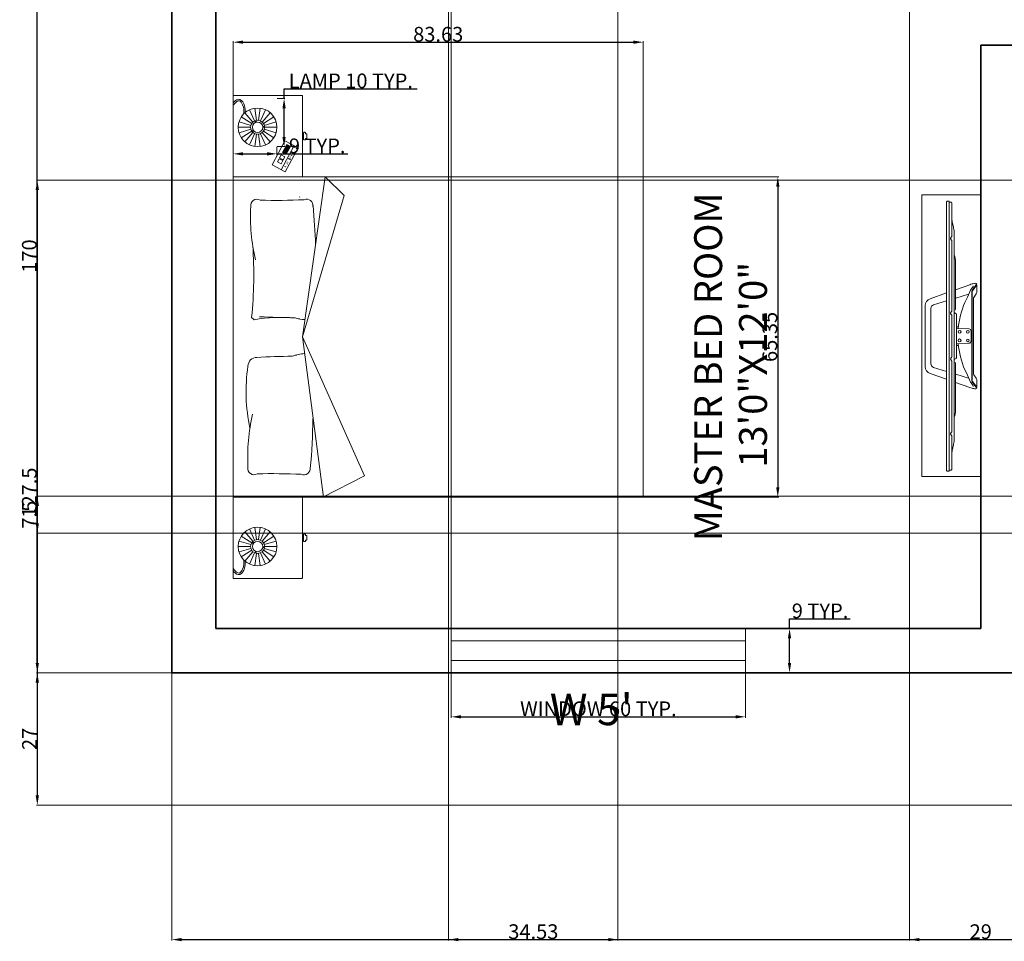
# Model space of a CAD drawing. Units: feet. Extents: x -297 to 770, y -228 to 625.
# Tile 1 of 14: x 351 to 552, y -228 to -40. Entities that reach past the tile are written whole.
import ezdxf

# ---------------------------------------------------------------- set-up
doc = ezdxf.new("R2010")
doc.units = ezdxf.units.FT
doc.header["$MEASUREMENT"] = 0
for name, color, linetype, lineweight in [('A-ANNO-DIMS', 2, 'Continuous', 18), ('A-ANNO-TEXT', 7, 'Continuous', 18), ('A-AREA-IDEN', 7, 'Continuous', 25), ('A-EQPM', 8, 'Continuous', 13), ('A-FURN', 8, 'Continuous', 18), ('A-WALL', 7, 'Continuous', 35), ('windows', 30, 'Continuous', 18)]:
    doc.layers.add(name, color=color, linetype=linetype, lineweight=lineweight)
doc.styles.add('Annotative', font='arial.ttf')
doc.styles.get("Standard").update_dxf_attribs({"font": 'arial.ttf'})
doc.dimstyles.get("Standard").update_dxf_attribs({"dimtxt": 3, "dimasz": 2, "dimexe": 0.18, "dimexo": 0.0625, "dimgap": 0.09, "dimtad": 1, "dimtoh": 1, "dimdec": 1, "dimzin": 0, "dimdsep": 46, "dimlunit": 3, "dimtxsty": 'Standard', "dimcen": 0, "dimclre": 256, "dimadec": 0, "dimazin": 0, "dimtfac": 1, "dimtdec": 1, "dimtofl": 0, "dimtmove": 0, "dimatfit": 3, "dimfxl": 1, "dimtolj": 1, "dimtzin": 0, "dimlwe": -1, "dimarcsym": 0})

# ---------------------------------------------------------------- blocks, each defined once
blk = doc.blocks.new('WIN-5FT')
for p, q in [((60, 6.5), (0, 6.5)), ((60, 2.5), (0, 2.5))]:
    blk.add_line(p, q)
blk.add_lwpolyline([(60, 0), (60, 9), (0, 9), (0, 0)], close=True)
blk = doc.blocks.new('LAMP-BEDSIDE')
for p, q in [((1.64, 6.07), (3.76, 4.71)), ((2.38, 6.92), (4.02, 5.02)), ((3.32, 7.53), (4.37, 5.24)), ((4.4, 7.84), (4.76, 5.35)), ((5.52, 7.84), (5.16, 5.35)), ((6.6, 7.53), (5.55, 5.24)), ((7.54, 6.92), (5.89, 5.02)), ((8.27, 6.07), (6.16, 4.71)), ((1.18, 5.05), (3.59, 4.34)), ((4.52, 4.9), (4.45, 5.28)), ((4.73, 4.97), (4.58, 5.32)), ((6, 4.13), (6.37, 4.13)), ((6.33, 4.34), (8.74, 5.05)), ((1.02, 3.94), (3.53, 3.94)), ((1.02, 3.94), (3.53, 3.94)), ((1.18, 2.83), (3.59, 3.54)), ((3.76, 3.17), (1.64, 1.81)), ((4.02, 2.86), (2.38, 0.96)), ((4.37, 2.64), (3.32, 0.36)), ((4.06, 3.38), (3.84, 3.06)), ((4.29, 3.12), (3.96, 2.92)), ((4.76, 2.53), (4.4, 0.04)), ((5.16, 2.53), (5.52, 0.04)), ((5.55, 2.64), (6.6, 0.36)), ((5.89, 2.86), (7.54, 0.96)), ((6.02, 3.89), (6.39, 3.98)), ((6.16, 3.17), (8.27, 1.81)), ((6.33, 3.54), (8.74, 2.83)), ((6.39, 3.94), (8.9, 3.94)), ((6.39, 3.94), (8.9, 3.94))]:
    blk.add_line(p, q)
for radius in [3.94, 1.43, 1.06]:
    blk.add_circle((4.96, 3.94), radius)
for points, knots in [([(2.46, 6.99), (2.46, 7.42), (2.45, 7.88), (2.14, 8.85), (1.91, 9.46), (0.86, 9.79), (0.47, 9.43), (0.1, 9.02), (0.05, 8.96), (0, 8.91)], [0.0077183, 0.0077183, 0.0077183, 0.0077183, 0.0428867, 0.0428867, 0.0785443, 0.0785443, 0.1084778, 0.1084778, 0.1132873, 0.1132873, 0.1132873, 0.1132873]), ([(2.16, 6.71), (2.17, 7.31), (2.19, 8.25), (1.15, 9.83), (0.43, 8.96), (0, 8.44)], [0, 0, 0, 0, 1.847824, 2.900884, 4.449581, 4.449581, 4.449581, 4.449581])]:
    blk.add_open_spline(points, degree=3, knots=knots)
blk = doc.blocks.new('*D19')
at = {"layer": 'A-ANNO-DIMS', "transparency": 16777216}
for p, q in [((439.16, -173.1), (439.16, -182.22)), ((499.16, -173.1), (499.16, -182.22))]:
    blk.add_line(p, q, dxfattribs=at)
at = {"layer": 'A-ANNO-DIMS', "color": 0, "lineweight": -2, "transparency": 16777216}
blk.add_line((441.16, -182.04), (497.16, -182.04), dxfattribs=at)
at = {"layer": 'A-ANNO-DIMS', "color": 0, "transparency": 16777216}
for points in [[(441.16, -181.7), (441.16, -182.37), (439.16, -182.04)], [(497.16, -181.7), (497.16, -182.37), (499.16, -182.04)]]:
    blk.add_solid(points, dxfattribs=at)
at = {"layer": 'Defpoints', "color": 0, "transparency": 16777216}
for p in [(439.16, -173.04), (499.16, -173.04), (499.16, -182.04)]:
    blk.add_point(p, dxfattribs=at)
at = {"layer": 'A-ANNO-DIMS', "color": 0, "transparency": 16777216, "insert": (469.16, -180.4), "char_height": 3, "attachment_point": 5}
blk.add_mtext('\\A1;WINDOW 60 TYP.', dxfattribs=at)
blk = doc.blocks.new('*D20')
at = {"layer": 'A-ANNO-DIMS', "color": 0, "lineweight": -2, "transparency": 16777216}
for p, q in [((508.16, -164.04), (508.16, -162.04)), ((508.16, -162.04), (520.52, -162.04)), ((508.16, -171.04), (508.16, -166.04))]:
    blk.add_line(p, q, dxfattribs=at)
at = {"layer": 'A-ANNO-DIMS', "transparency": 16777216}
for p, q in [((499.22, -164.04), (508.34, -164.04)), ((499.22, -173.04), (508.34, -173.04))]:
    blk.add_line(p, q, dxfattribs=at)
at = {"layer": 'A-ANNO-DIMS', "color": 0, "transparency": 16777216}
for points in [[(507.82, -166.04), (508.49, -166.04), (508.16, -164.04)], [(507.82, -171.04), (508.49, -171.04), (508.16, -173.04)]]:
    blk.add_solid(points, dxfattribs=at)
at = {"layer": 'Defpoints', "color": 0, "transparency": 16777216}
for p in [(499.16, -164.04), (508.16, -164.04), (499.16, -173.04)]:
    blk.add_point(p, dxfattribs=at)
at = {"layer": 'A-ANNO-DIMS', "color": 0, "transparency": 16777216, "insert": (514.38, -160.42), "char_height": 3, "attachment_point": 5}
blk.add_mtext('\\A1;9 TYP.', dxfattribs=at)
blk = doc.blocks.new('*D25')
at = {"layer": 'A-ANNO-DIMS', "color": 0, "lineweight": -2, "transparency": 16777216}
for p, q in [((405.05, -55.92), (405.05, -53.92)), ((405.05, -53.92), (432.18, -53.92)), ((405.05, -63.72), (405.05, -57.92))]:
    blk.add_line(p, q, dxfattribs=at)
at = {"layer": 'A-ANNO-DIMS', "transparency": 16777216}
for p, q in [((403.64, -55.92), (405.23, -55.92)), ((403.64, -65.72), (405.23, -65.72))]:
    blk.add_line(p, q, dxfattribs=at)
at = {"layer": 'A-ANNO-DIMS', "color": 0, "transparency": 16777216}
for points in [[(404.71, -57.92), (405.38, -57.92), (405.05, -55.92)], [(404.71, -63.72), (405.38, -63.72), (405.05, -65.72)]]:
    blk.add_solid(points, dxfattribs=at)
at = {"layer": 'Defpoints', "color": 0, "transparency": 16777216}
for p in [(403.58, -55.92), (405.05, -55.92), (403.58, -65.72)]:
    blk.add_point(p, dxfattribs=at)
at = {"layer": 'A-ANNO-DIMS', "color": 0, "transparency": 16777216, "insert": (418.66, -52.3), "char_height": 3, "attachment_point": 5}
blk.add_mtext('\\A1;LAMP 10 TYP.', dxfattribs=at)
blk = doc.blocks.new('*D26')
at = {"layer": 'A-ANNO-DIMS', "transparency": 16777216}
for p, q in [((394.68, -65.78), (394.68, -67.37)), ((403.58, -65.78), (403.58, -67.37))]:
    blk.add_line(p, q, dxfattribs=at)
at = {"layer": 'A-ANNO-DIMS', "color": 0, "lineweight": -2, "transparency": 16777216}
for p, q in [((396.68, -67.19), (401.58, -67.19)), ((403.58, -67.19), (418.03, -67.19))]:
    blk.add_line(p, q, dxfattribs=at)
at = {"layer": 'A-ANNO-DIMS', "color": 0, "transparency": 16777216}
for points in [[(396.68, -66.85), (396.68, -67.52), (394.68, -67.19)], [(401.58, -66.85), (401.58, -67.52), (403.58, -67.19)]]:
    blk.add_solid(points, dxfattribs=at)
at = {"layer": 'Defpoints', "color": 0, "transparency": 16777216}
for p in [(394.68, -65.72), (403.58, -65.72), (403.58, -67.19)]:
    blk.add_point(p, dxfattribs=at)
at = {"layer": 'A-ANNO-DIMS', "color": 0, "transparency": 16777216, "insert": (411.8, -65.56), "char_height": 3, "attachment_point": 5}
blk.add_mtext('\\A1;9 TYP.', dxfattribs=at)
blk = doc.blocks.new('*D43')
at = {"layer": 'A-ANNO-DIMS', "transparency": 16777216}
for p, q in [((382.16, -173.1), (382.16, -227.67)), ((742.16, -200.1), (742.16, -227.67))]:
    blk.add_line(p, q, dxfattribs=at)
at = {"layer": 'A-ANNO-DIMS', "color": 0, "lineweight": -2, "transparency": 16777216}
blk.add_line((384.16, -227.49), (740.16, -227.49), dxfattribs=at)
at = {"layer": 'A-ANNO-DIMS', "color": 0, "transparency": 16777216}
for points in [[(384.16, -227.15), (384.16, -227.82), (382.16, -227.49)], [(740.16, -227.15), (740.16, -227.82), (742.16, -227.49)]]:
    blk.add_solid(points, dxfattribs=at)
at = {"layer": 'Defpoints', "color": 0, "transparency": 16777216}
for p in [(382.16, -173.04), (742.16, -200.04), (742.16, -227.49)]:
    blk.add_point(p, dxfattribs=at)
at = {"layer": 'A-ANNO-DIMS', "color": 0, "transparency": 16777216, "insert": (562.16, -225.86), "char_height": 3, "attachment_point": 5}
blk.add_mtext('\\A1;360', dxfattribs=at)
blk = doc.blocks.new('*D45')
at = {"layer": 'A-ANNO-DIMS', "transparency": 16777216}
for p, q in [((382.09, -173.04), (354.53, -173.04)), ((556.09, -200.04), (354.53, -200.04))]:
    blk.add_line(p, q, dxfattribs=at)
at = {"layer": 'A-ANNO-DIMS', "color": 0, "lineweight": -2, "transparency": 16777216}
blk.add_line((354.71, -175.04), (354.71, -198.04), dxfattribs=at)
at = {"layer": 'A-ANNO-DIMS', "color": 0, "transparency": 16777216}
for points in [[(354.37, -175.04), (355.04, -175.04), (354.71, -173.04)], [(354.37, -198.04), (355.04, -198.04), (354.71, -200.04)]]:
    blk.add_solid(points, dxfattribs=at)
at = {"layer": 'Defpoints', "color": 0, "transparency": 16777216}
for p in [(382.16, -173.04), (354.71, -200.04), (556.16, -200.04)]:
    blk.add_point(p, dxfattribs=at)
at = {"layer": 'A-ANNO-DIMS', "color": 0, "transparency": 16777216, "insert": (353.11, -186.54), "char_height": 3, "attachment_point": 5, "rotation": 90}
blk.add_mtext('\\A1;27', dxfattribs=at)
blk = doc.blocks.new('*D53')
at = {"layer": 'A-ANNO-DIMS', "transparency": 16777216}
for p, q in [((382.09, -3.04), (354.53, -3.04)), ((382.09, -173.04), (354.53, -173.04))]:
    blk.add_line(p, q, dxfattribs=at)
at = {"layer": 'A-ANNO-DIMS', "color": 0, "lineweight": -2, "transparency": 16777216}
blk.add_line((354.71, -171.04), (354.71, -5.04), dxfattribs=at)
at = {"layer": 'A-ANNO-DIMS', "color": 0, "transparency": 16777216}
for points in [[(354.37, -5.04), (355.04, -5.04), (354.71, -3.04)], [(354.37, -171.04), (355.04, -171.04), (354.71, -173.04)]]:
    blk.add_solid(points, dxfattribs=at)
at = {"layer": 'Defpoints', "color": 0, "transparency": 16777216}
for p in [(354.71, -3.04), (382.16, -3.04), (382.16, -173.04)]:
    blk.add_point(p, dxfattribs=at)
at = {"layer": 'A-ANNO-DIMS', "color": 0, "transparency": 16777216, "insert": (353.08, -88.04), "char_height": 3, "attachment_point": 5, "rotation": 90}
blk.add_mtext('\\A1;170', dxfattribs=at)
blk = doc.blocks.new('*D56')
at = {"layer": 'A-ANNO-DIMS', "transparency": 16777216}
for p, q in [((742.09, -72.54), (354.53, -72.54)), ((742.09, -200.04), (354.53, -200.04))]:
    blk.add_line(p, q, dxfattribs=at)
at = {"layer": 'A-ANNO-DIMS', "color": 0, "lineweight": -2, "transparency": 16777216}
blk.add_line((354.71, -74.54), (354.71, -198.04), dxfattribs=at)
at = {"layer": 'A-ANNO-DIMS', "color": 0, "transparency": 16777216}
for points in [[(354.37, -74.54), (355.04, -74.54), (354.71, -72.54)], [(354.37, -198.04), (355.04, -198.04), (354.71, -200.04)]]:
    blk.add_solid(points, dxfattribs=at)
at = {"layer": 'Defpoints', "color": 0, "transparency": 16777216}
for p in [(742.16, -72.54), (354.71, -200.04), (742.16, -200.04)]:
    blk.add_point(p, dxfattribs=at)
at = {"layer": 'A-ANNO-DIMS', "color": 0, "transparency": 16777216, "insert": (353.08, -136.29), "char_height": 3, "attachment_point": 5, "rotation": 90}
blk.add_mtext('\\A1;127.5', dxfattribs=at)
blk = doc.blocks.new('*D57')
at = {"layer": 'A-ANNO-DIMS', "transparency": 16777216}
for p, q in [((391.16, -163.97), (391.16, 367.22)), ((439.16, -163.97), (439.16, 367.22))]:
    blk.add_line(p, q, dxfattribs=at)
at = {"layer": 'A-ANNO-DIMS', "color": 0, "lineweight": -2, "transparency": 16777216}
blk.add_line((393.16, 367.04), (437.16, 367.04), dxfattribs=at)
at = {"layer": 'A-ANNO-DIMS', "color": 0, "transparency": 16777216}
for points in [[(393.16, 367.38), (393.16, 366.71), (391.16, 367.04)], [(437.16, 367.38), (437.16, 366.71), (439.16, 367.04)]]:
    blk.add_solid(points, dxfattribs=at)
at = {"layer": 'Defpoints', "color": 0, "transparency": 16777216}
for p in [(439.16, 367.04), (391.16, -164.04), (439.16, -164.04)]:
    blk.add_point(p, dxfattribs=at)
at = {"layer": 'A-ANNO-DIMS', "color": 0, "transparency": 16777216, "insert": (415.16, 368.66), "char_height": 3, "attachment_point": 5}
blk.add_mtext('\\A1;48', dxfattribs=at)
blk = doc.blocks.new('*D59')
at = {"layer": 'A-ANNO-DIMS', "transparency": 16777216}
for p, q in [((652.09, -137.04), (354.53, -137.04)), ((652.09, -144.54), (354.53, -144.54))]:
    blk.add_line(p, q, dxfattribs=at)
at = {"layer": 'A-ANNO-DIMS', "color": 0, "lineweight": -2, "transparency": 16777216}
blk.add_line((354.71, -142.54), (354.71, -139.04), dxfattribs=at)
at = {"layer": 'A-ANNO-DIMS', "color": 0, "transparency": 16777216}
for points in [[(354.37, -139.04), (355.04, -139.04), (354.71, -137.04)], [(354.37, -142.54), (355.04, -142.54), (354.71, -144.54)]]:
    blk.add_solid(points, dxfattribs=at)
at = {"layer": 'Defpoints', "color": 0, "transparency": 16777216}
for p in [(354.71, -137.04), (652.16, -137.04), (652.16, -144.54)]:
    blk.add_point(p, dxfattribs=at)
at = {"layer": 'A-ANNO-DIMS', "color": 0, "transparency": 16777216, "insert": (353.09, -140.79), "char_height": 3, "attachment_point": 5, "rotation": 90}
blk.add_mtext('\\A1;7.5', dxfattribs=at)
blk = doc.blocks.new('*D67')
at = {"layer": 'A-ANNO-DIMS', "transparency": 16777216}
for p, q in [((532.66, 197.4), (532.66, -227.67)), ((561.66, 197.4), (561.66, -227.67))]:
    blk.add_line(p, q, dxfattribs=at)
at = {"layer": 'A-ANNO-DIMS', "color": 0, "lineweight": -2, "transparency": 16777216}
blk.add_line((534.66, -227.49), (559.66, -227.49), dxfattribs=at)
at = {"layer": 'A-ANNO-DIMS', "color": 0, "transparency": 16777216}
for points in [[(534.66, -227.15), (534.66, -227.82), (532.66, -227.49)], [(559.66, -227.15), (559.66, -227.82), (561.66, -227.49)]]:
    blk.add_solid(points, dxfattribs=at)
at = {"layer": 'Defpoints', "color": 0, "transparency": 16777216}
for p in [(532.66, 197.46), (561.66, 197.46), (561.66, -227.49)]:
    blk.add_point(p, dxfattribs=at)
at = {"layer": 'A-ANNO-DIMS', "color": 0, "transparency": 16777216, "insert": (547.16, -225.87), "char_height": 3, "attachment_point": 5}
blk.add_mtext('\\A1;29', dxfattribs=at)
blk = doc.blocks.new('*D69')
at = {"layer": 'A-ANNO-DIMS', "transparency": 16777216}
for p, q in [((438.62, -20.1), (438.62, -227.67)), ((473.16, -20.1), (473.16, -227.67))]:
    blk.add_line(p, q, dxfattribs=at)
at = {"layer": 'A-ANNO-DIMS', "color": 0, "lineweight": -2, "transparency": 16777216}
blk.add_line((440.62, -227.49), (471.16, -227.49), dxfattribs=at)
at = {"layer": 'A-ANNO-DIMS', "color": 0, "transparency": 16777216}
for points in [[(440.62, -227.15), (440.62, -227.82), (438.62, -227.49)], [(471.16, -227.15), (471.16, -227.82), (473.16, -227.49)]]:
    blk.add_solid(points, dxfattribs=at)
at = {"layer": 'Defpoints', "color": 0, "transparency": 16777216}
for p in [(438.62, -20.04), (473.16, -20.04), (473.16, -227.49)]:
    blk.add_point(p, dxfattribs=at)
at = {"layer": 'A-ANNO-DIMS', "color": 0, "transparency": 16777216, "insert": (455.89, -225.86), "char_height": 3, "attachment_point": 5}
blk.add_mtext('\\A1;34.53', dxfattribs=at)
blk = doc.blocks.new('*D78')
at = {"layer": 'A-ANNO-DIMS', "transparency": 16777216}
for p, q in [((394.68, -71.8), (394.68, -44.23)), ((478.31, -71.8), (478.31, -44.23))]:
    blk.add_line(p, q, dxfattribs=at)
at = {"layer": 'A-ANNO-DIMS', "color": 0, "lineweight": -2, "transparency": 16777216}
blk.add_line((396.68, -44.41), (476.31, -44.41), dxfattribs=at)
at = {"layer": 'A-ANNO-DIMS', "color": 0, "transparency": 16777216}
for points in [[(396.68, -44.08), (396.68, -44.74), (394.68, -44.41)], [(476.31, -44.08), (476.31, -44.74), (478.31, -44.41)]]:
    blk.add_solid(points, dxfattribs=at)
at = {"layer": 'Defpoints', "color": 0, "transparency": 16777216}
for p in [(478.31, -44.41), (394.68, -71.86), (478.31, -71.86)]:
    blk.add_point(p, dxfattribs=at)
at = {"layer": 'A-ANNO-DIMS', "color": 0, "transparency": 16777216, "insert": (436.49, -42.79), "char_height": 3, "attachment_point": 5}
blk.add_mtext('\\A1;83.63', dxfattribs=at)
blk = doc.blocks.new('*D79')
at = {"layer": 'A-ANNO-DIMS', "transparency": 16777216}
for p, q in [((478.37, -71.86), (505.94, -71.86)), ((478.37, -137.21), (505.94, -137.21))]:
    blk.add_line(p, q, dxfattribs=at)
at = {"layer": 'A-ANNO-DIMS', "color": 0, "lineweight": -2, "transparency": 16777216}
blk.add_line((505.76, -73.86), (505.76, -135.21), dxfattribs=at)
at = {"layer": 'A-ANNO-DIMS', "color": 0, "transparency": 16777216}
for points in [[(505.43, -73.86), (506.09, -73.86), (505.76, -71.86)], [(505.43, -135.21), (506.09, -135.21), (505.76, -137.21)]]:
    blk.add_solid(points, dxfattribs=at)
at = {"layer": 'Defpoints', "color": 0, "transparency": 16777216}
for p in [(478.31, -71.86), (478.31, -137.21), (505.76, -137.21)]:
    blk.add_point(p, dxfattribs=at)
at = {"layer": 'A-ANNO-DIMS', "color": 0, "transparency": 16777216, "insert": (504.14, -104.54), "char_height": 3, "attachment_point": 5, "rotation": 90}
blk.add_mtext('\\A1;65.35', dxfattribs=at)

msp = doc.modelspace()

# ---------------------------------------------------------------- linework, layer by layer
at = {"layer": 'A-EQPM'}
for p, q in [((540.182, -76.989), (540.182, -104.393)), ((540.707, -77.028), (540.707, -104.372)), ((541.083, -84.682), (541.083, -84.213)), ((541.733, -83.09), (541.733, -104.372)), ((541.083, -99.931), (541.083, -99.463)), ((540.182, -131.755), (540.182, -104.351)), ((540.707, -131.716), (540.707, -104.372)), ((541.733, -125.654), (541.733, -104.372)), ((541.083, -108.812), (541.083, -109.281)), ((541.083, -124.062), (541.083, -124.531))]:
    msp.add_line(p, q, dxfattribs=at)
for points in [[(540.707, -77.028), (540.707, -76.832), (540.339, -76.832)], [(541.113, -77.028), (540.707, -77.028)], [(541.27, -80.413), (541.27, -83.91)], [(541.27, -84.985), (541.27, -99.159)], [(542.014, -96.619), (542.079, -96.599)], [(541.27, -100.235), (541.27, -104.372)], [(541.27, -108.509), (541.27, -104.372)], [(542.596, -102.489), (542.189, -102.457)], [(542.596, -106.255), (542.189, -106.287)], [(541.27, -123.759), (541.27, -109.584)], [(542.014, -112.125), (542.079, -112.144)], [(541.27, -128.331), (541.27, -124.834)], [(540.707, -131.716), (540.707, -131.912), (540.339, -131.912)], [(541.113, -131.716), (540.707, -131.716)]]:
    msp.add_lwpolyline(points, dxfattribs=at)
for points in [[(541.733, -83.09, 0.0321699), (541.581, -82.109, 0.0029358), (541.397, -81.299, -0.0437499), (541.27, -80.413), (541.27, -77.184)], [(541.021, -84.447), (541.021, -84.387, -0.2123222), (541.111, -84.184, 0.0857419), (541.239, -84.021, 0.1124025), (541.27, -83.91, 5.368)], [(541.021, -84.447), (541.021, -84.508, 0.2123222), (541.111, -84.711, -0.0857419), (541.239, -84.874, -0.1124025), (541.27, -84.985, -5.368)], [(542.014, -96.678), (542.014, -89.258, 0.0958514), (541.733, -87.806, 2.9419791)], [(545.654, -104.372), (545.654, -96.676, -0.1606369), (545.718, -96.484), (546.25, -95.762, 0.1675007), (546.331, -95.502), (546.331, -93.927, -0.0429709), (546.302, -93.877), (546.302, -93.877, -0.095732), (546.28, -93.805, 0.3452993), (546.268, -93.672, 0.2278474), (546.056, -93.604, 0.0317538), (545.405, -93.735, 0.0183529), (544.911, -93.887), (542.014, -94.916)], [(542.556, -102.81), (542.636, -102.168, -0.0837977), (544.23, -96.865, 0.0073252), (545.093, -95.003), (545.093, -95.003, -0.0079676), (545.596, -94.238, 0.3265331), (545.584, -94.085)], [(546.28, -93.805), (545.389, -95.071, 0.1365415), (545.309, -95.297), (545.309, -104.372)], [(546.331, -93.927), (545.481, -95.136, 0.1337651), (545.422, -95.301), (545.422, -104.372)], [(540.182, -95.567), (536.831, -96.757, 0.3109471), (535.819, -98.154), (535.819, -104.372)], [(542.079, -96.599, -0.0518689), (542.079, -96.599), (544.64, -95.805, -0.3772566), (544.713, -95.838)], [(536.979, -104.372), (536.979, -98.75, -0.3044482), (537.506, -97.965), (540.182, -97.166)], [(541.733, -99.045), (541.808, -99.045, 0.3443306), (542.014, -98.883), (542.014, -96.678)], [(541.021, -99.697), (541.021, -99.636, -0.2123222), (541.111, -99.434, 0.0857419), (541.239, -99.27, 0.1124025), (541.27, -99.159, 5.368)], [(541.021, -99.697), (541.021, -99.758, 0.2123222), (541.111, -99.961, -0.0857419), (541.239, -100.124, -0.1124025), (541.27, -100.235, -5.368)], [(542.189, -104.372), (542.189, -99.927, 0.2006899), (542.149, -99.832), (541.849, -99.654), (541.733, -99.654)], [(540.182, -113.177), (536.831, -111.987, -0.3109471), (535.819, -110.589), (535.819, -104.372)], [(536.979, -104.372), (536.979, -109.994, 0.3044482), (537.506, -110.779), (540.182, -111.578)], [(542.189, -104.372), (542.189, -108.817, -0.2006899), (542.149, -108.912), (541.849, -109.09), (541.733, -109.09)], [(545.654, -104.372), (545.654, -112.068, 0.1606369), (545.718, -112.259), (546.25, -112.982, -0.1675007), (546.331, -113.242), (546.331, -114.816, 0.0429709), (546.302, -114.867), (546.302, -114.867, 0.095732), (546.28, -114.939, -0.3452993), (546.268, -115.072, -0.2278474), (546.056, -115.14, -0.0317538), (545.405, -115.009, -0.0183529), (544.911, -114.857), (542.014, -113.828)], [(545.175, -104.372), (545.175, -104.372), (545.175, -103.381, 0.4039521), (544.752, -102.903), (542.189, -102.794)], [(545.175, -104.372), (545.175, -104.372), (545.175, -105.362, -0.4039521), (544.752, -105.841), (542.189, -105.949)], [(546.28, -114.939), (545.389, -113.673, -0.1365415), (545.309, -113.447), (545.309, -104.372)], [(546.331, -114.816), (545.481, -113.608, -0.1337651), (545.422, -113.443), (545.422, -104.372)], [(542.556, -105.934), (542.636, -106.576, 0.0837977), (544.23, -111.879, -0.0073252), (545.093, -113.741), (545.093, -113.741, 0.0079676), (545.596, -114.506, -0.3265331), (545.584, -114.659)], [(541.021, -109.047), (541.021, -108.986, -0.2123222), (541.111, -108.783, 0.0857419), (541.239, -108.62, 0.1124025), (541.27, -108.509, 5.368)], [(541.021, -109.047), (541.021, -109.107, 0.2123222), (541.111, -109.31, -0.0857419), (541.239, -109.473, -0.1124025), (541.27, -109.584, -5.368)], [(541.733, -109.699), (541.808, -109.699, -0.3443306), (542.014, -109.861), (542.014, -112.066)], [(542.014, -112.066), (542.014, -119.485, -0.0958514), (541.733, -120.937, -2.9419791)], [(542.079, -112.144, 0.0518689), (542.079, -112.144), (544.64, -112.939, 0.3772566), (544.713, -112.906)], [(541.021, -124.296), (541.021, -124.236, -0.2123222), (541.111, -124.033, 0.0857419), (541.239, -123.87, 0.1124025), (541.27, -123.759, 5.368)], [(541.021, -124.296), (541.021, -124.357, 0.2123222), (541.111, -124.56, -0.0857419), (541.239, -124.723, -0.1124025), (541.27, -124.834, -5.368)], [(541.733, -125.654, -0.0321699), (541.581, -126.635, -0.0029358), (541.397, -127.445, 0.0437499), (541.27, -128.331), (541.27, -131.559)]]:
    msp.add_lwpolyline(points, format="xyb", dxfattribs=at)
for centre, radius in [((542.833, -103.5), 0.3), ((544.546, -103.5), 0.27), ((542.833, -105.244), 0.3), ((544.546, -105.244), 0.27)]:
    msp.add_circle(centre, radius, dxfattribs=at)
for centre, start, end in [((540.339, -76.989), 90, 180), ((541.113, -77.184), 0, 90), ((540.339, -131.755), 180, 270), ((541.113, -131.559), 270, 0)]:
    msp.add_arc(centre, 0.157, start, end, dxfattribs=at)
at = {"layer": 'A-FURN'}
for p, q in [((394.677, -71.861), (394.677, -55.269)), ((394.677, -55.269), (408.691, -55.269)), ((394.677, -71.861), (394.677, -55.269)), ((408.778, -55.355), (408.778, -71.775)), ((408.778, -63.856), (408.778, -63.274)), ((408.778, -63.274), (409.024, -63.274)), ((409.024, -63.856), (408.778, -63.856)), ((409.024, -64.265), (409.024, -62.864)), ((409.111, -62.778), (409.303, -62.778)), ((409.389, -62.864), (409.389, -63.017)), ((409.619, -64.026), (409.389, -64.026)), ((409.389, -64.026), (409.389, -64.265)), ((409.476, -63.104), (409.619, -63.104)), ((409.705, -63.19), (409.705, -63.94)), ((402.614, -69.453), (405.232, -64.514)), ((404.457, -70.43), (407.075, -65.491)), ((405.588, -65.257), (404.724, -66.887)), ((405.677, -65.304), (404.813, -66.935)), ((405.82, -65.38), (404.956, -67.011)), ((405.923, -65.434), (405.058, -67.065)), ((406.012, -65.482), (405.148, -67.112)), ((406.089, -65.523), (405.225, -67.153)), ((405.232, -64.514), (407.91, -65.934)), ((407.91, -65.934), (405.292, -70.872)), ((406.21, -65.587), (405.346, -67.217)), ((406.342, -65.657), (405.477, -67.287)), ((405.588, -65.257), (406.342, -65.657)), ((409.303, -64.352), (409.111, -64.352)), ((403.709, -68.801), (404.04, -68.176)), ((404.04, -68.176), (404.794, -68.576)), ((404.136, -67.997), (404.467, -67.373)), ((404.889, -68.397), (404.136, -67.997)), ((404.467, -67.373), (405.22, -67.772)), ((405.477, -67.287), (404.724, -66.887)), ((405.22, -67.772), (404.889, -68.397)), ((405.292, -70.872), (402.614, -69.453)), ((404.463, -69.2), (403.709, -68.801)), ((404.794, -68.576), (404.463, -69.2)), ((394.677, -137.214), (394.677, -71.861)), ((394.677, -71.861), (478.31, -71.861)), ((408.783, -104.537), (413.455, -71.861)), ((413.455, -71.861), (417.276, -75.689)), ((478.31, -71.861), (478.31, -137.214)), ((417.276, -75.689), (408.783, -104.537)), ((547.155, -75.537), (535.155, -75.537)), ((535.155, -75.537), (535.155, -133.037)), ((547.155, -133.037), (547.155, -75.537)), ((394.677, -137.214), (394.677, -104.537)), ((421.451, -132.909), (408.783, -104.537)), ((408.783, -104.537), (413.067, -137.214)), ((412.961, -137.214), (421.451, -132.909)), ((535.155, -133.037), (547.155, -133.037)), ((478.31, -137.214), (394.677, -137.214)), ((394.677, -137.214), (394.677, -153.806)), ((394.677, -137.214), (394.677, -153.806)), ((394.677, -137.214), (408.691, -137.214)), ((408.778, -153.719), (408.778, -137.3)), ((409.024, -145.219), (408.778, -145.219)), ((408.778, -145.219), (408.778, -145.801)), ((408.778, -145.801), (409.024, -145.801)), ((409.024, -144.809), (409.024, -146.21)), ((409.303, -144.723), (409.111, -144.723)), ((409.111, -146.296), (409.303, -146.296)), ((409.389, -145.048), (409.389, -144.809)), ((409.619, -145.048), (409.389, -145.048)), ((409.389, -146.21), (409.389, -146.057)), ((409.476, -145.971), (409.619, -145.971)), ((409.705, -145.885), (409.705, -145.135)), ((394.677, -153.806), (408.691, -153.806))]:
    msp.add_line(p, q, dxfattribs=at)
for centre, radius, start, end in [((408.691, -55.355), 0.0863, 0, 90), ((409.111, -62.864), 0.0863, 90, 180), ((409.111, -64.265), 0.0863, 180, 270), ((409.303, -62.864), 0.0863, 0, 90), ((409.303, -64.265), 0.0863, 270, 0), ((409.476, -63.017), 0.0863, 180, 270), ((409.619, -63.19), 0.0863, 0, 90), ((409.619, -63.94), 0.0863, 270, 0), ((407.273, -65.855), 0.0506, 0, 180), ((407.273, -65.855), 0.0506, 180, 0), ((407.592, -66.037), 0.0506, 0, 180), ((407.592, -66.037), 0.0506, 180, 0), ((406.024, -68.16), 0.0506, 0, 180), ((406.024, -68.16), 0.0506, 180, 0), ((406.28, -68.317), 0.0506, 0, 180), ((406.28, -68.317), 0.0506, 180, 0), ((408.166, -75.973), 0.069, 270, 0), ((437.376, -80.042), 39.175, 176.95117, 192.94362), ((437.376, -80.042), 39.175, 176.95117, 192.94362), ((399.49, -77.713), 1.258, 58.3905, 191.27221), ((399.49, -77.713), 1.258, 58.3905, 191.27221), ((403.323, 52.874), 129.555, 268.59625, 272.56667), ((403.323, 52.874), 129.555, 268.59625, 272.56667), ((409.652, -77.741), 1.301, 350.34242, 113.89159), ((409.652, -77.741), 1.301, 350.34242, 113.89159), ((310.662, -88.08), 100.822, 1.28421, 5.88609), ((310.662, -88.08), 100.822, 1.28421, 5.88609), ((315.255, -91.953), 83.612, 354.09622, 4.11018), ((400.002, -99.31), 2.01, 131.3461, 131.8512), ((410.722, 114.833), 215.502, 267.16594, 269.08744), ((400.002, -99.31), 2.01, 218.22652, 238.49477), ((404.733, -136.117), 35.567, 85.87807, 99.3556), ((408.36, -98.28), 2.594, 245.62563, 267.33023), ((409.084, -95.927), 5.045, 249.16323, 272.37479), ((410.379, -119.254), 11.392, 95.86257, 108.75888), ((407.786, -110.83), 2.594, 92.66977, 114.37437), ((399.493, -110.513), 1.81, 90, 180), ((399.493, -110.513), 1.81, 90, 180), ((410.148, -323.942), 215.502, 90.91256, 92.83406), ((410.148, -323.942), 215.502, 90.91256, 92.83406), ((432.589, -115.748), 35.296, 171.47023, 192.10326), ((432.589, -115.748), 35.296, 171.47023, 192.10326), ((436.802, -129.067), 39.175, 167.05638, 183.04883), ((436.802, -129.067), 39.175, 167.05638, 183.04883), ((310.089, -121.03), 100.822, 354.11391, 359.91574), ((310.089, -121.03), 100.822, 354.11391, 359.91574), ((398.916, -131.397), 1.258, 168.72779, 301.6095), ((398.916, -131.397), 1.258, 168.72779, 301.6095), ((402.749, -261.983), 129.555, 87.43333, 91.40375), ((402.749, -261.983), 129.555, 87.43333, 91.40375), ((409.078, -131.369), 1.301, 246.10841, 9.65758), ((409.078, -131.369), 1.301, 246.10841, 9.65758), ((409.111, -144.809), 0.0863, 90, 180), ((409.111, -146.21), 0.0863, 180, 270), ((409.303, -144.809), 0.0863, 0, 90), ((409.303, -146.21), 0.0863, 270, 0), ((409.476, -146.057), 0.0863, 90, 180), ((409.619, -145.135), 0.0863, 0, 90), ((409.619, -145.885), 0.0863, 270, 0), ((408.691, -153.719), 0.0863, 270, 0)]:
    msp.add_arc(centre, radius, start, end, dxfattribs=at)
at = {"layer": 'A-WALL'}
for p, q in [((391.155, -20.037), (391.155, -164.037)), ((547.155, -164.037), (547.155, -45.037)), ((547.155, -45.037), (556.155, -45.037)), ((391.155, -164.037), (547.155, -164.037))]:
    msp.add_line(p, q, dxfattribs=at)
msp.add_lwpolyline([(685.155, 306.963), (382.155, 306.963), (382.155, -173.037), (556.155, -173.037)], dxfattribs=at)

# ---------------------------------------------------------------- block references
at = {"layer": 'A-FURN'}
msp.add_blockref('LAMP-BEDSIDE', (394.677, -65.717), dxfattribs=at)
at = {"layer": 'A-FURN', "extrusion": (0, 0, -1), "zscale": -1, "rotation": 180}
msp.add_blockref('LAMP-BEDSIDE', (-394.677, -143.358), dxfattribs=at)
at = {"layer": 'windows'}
msp.add_blockref('WIN-5FT', (439.155, -173.037), dxfattribs=at)

# ---------------------------------------------------------------- texts
at = {"layer": 'A-ANNO-TEXT', "style": 'Annotative'}
msp.add_text("W 5'", height=6.4048, dxfattribs=at).set_placement((459.256, -183.744))
at = {"layer": 'A-AREA-IDEN', "style": 'Annotative'}
for s, p in [('MASTER BED ROOM', (494.404, -146.214)), ('13\'0"X12\'0"', (503.554, -131.207))]:
    msp.add_text(s, height=5.69601, rotation=90, dxfattribs=at).set_placement(p)
at = {"layer": 'A-FURN', "width": 3}
msp.add_text('12 00', height=0.3613, rotation=60.64352, dxfattribs=at).set_placement((405.243, -70.208))

# ---------------------------------------------------------------- dimensions: what is measured, and where the dimension line sits
at = {"layer": 'A-ANNO-DIMS'}
for base, p1, p2, override, picture, middle in [((439.155, 367.042), (391.155, -164.037), (439.155, -164.037), {"dimdec": 0, "dimlfac": 1, "dimrnd": 0, "dimzin": 0, "dimdsep": 46, "dimlunit": 2}, '*D57', (415.155, 368.664)), ((561.655, -227.487), (532.655, 197.463), (561.655, 197.463), {"dimdec": 0, "dimlfac": 1, "dimrnd": 0, "dimzin": 0, "dimdsep": 46, "dimlunit": 2}, '*D67', (547.155, -225.866)), ((473.155, -227.487), (438.624, -20.037), (473.155, -20.041), {"dimdec": 2, "dimlfac": 1, "dimrnd": 0, "dimzin": 0, "dimdsep": 46, "dimlunit": 2}, '*D69', (455.889, -225.865)), ((478.31, -44.411), (394.677, -71.861), (478.31, -71.861), {"dimdec": 2, "dimlfac": 1, "dimrnd": 0, "dimzin": 0, "dimdsep": 46, "dimlunit": 2}, '*D78', (436.494, -42.788)), ((742.155, -227.487), (382.155, -173.037), (742.155, -200.037), {"dimdec": 0, "dimlfac": 1, "dimrnd": 0, "dimzin": 0, "dimdsep": 46, "dimlunit": 2}, '*D43', (562.155, -225.865))]:
    dim = msp.add_linear_dim(base=base, p1=p1, p2=p2, dimstyle='Standard', override=override, dxfattribs=at)
    dim.commit()
    dim.dimension.update_dxf_attribs({"geometry": picture, "text_midpoint": middle})
for base, p1, p2, angle, override, picture, middle in [((354.705, -3.037), (382.155, -173.037), (382.155, -3.037), 90, {"dimdec": 0, "dimlfac": 1, "dimrnd": 0, "dimzin": 0, "dimdsep": 46, "dimlunit": 2}, '*D53', (353.084, -88.037)), ((505.76, -137.214), (478.31, -71.861), (478.31, -137.214), 270, {"dimdec": 2, "dimlfac": 1, "dimrnd": 0, "dimzin": 0, "dimdsep": 46, "dimlunit": 2}, '*D79', (504.138, -104.537)), ((354.705, -200.037), (742.155, -72.537), (742.155, -200.037), 90, {"dimdec": 1, "dimlfac": 1, "dimrnd": 0, "dimzin": 0, "dimdsep": 46, "dimlunit": 2}, '*D56', (353.084, -136.287)), ((354.705, -137.037), (652.155, -144.537), (652.155, -137.037), 90, {"dimdec": 1, "dimlfac": 1, "dimrnd": 0, "dimzin": 0, "dimdsep": 46, "dimlunit": 2}, '*D59', (353.09, -140.787)), ((354.705, -200.037), (382.155, -173.037), (556.155, -200.037), 90, {"dimdec": 0, "dimlfac": 1, "dimrnd": 0, "dimzin": 0, "dimdsep": 46, "dimlunit": 2}, '*D45', (353.109, -186.537))]:
    dim = msp.add_linear_dim(base=base, p1=p1, p2=p2, angle=angle, dimstyle='Standard', override=override, dxfattribs=at)
    dim.commit()
    dim.dimension.update_dxf_attribs({"geometry": picture, "text_midpoint": middle})
for base, p1, p2, text, picture, middle in [((405.046, -55.922), (403.577, -65.717), (403.577, -55.922), 'LAMP <> TYP.', '*D25', (418.66, -52.3)), ((508.155, -164.037), (499.155, -173.037), (499.155, -164.037), '<> TYP.', '*D20', (514.381, -160.416))]:
    dim = msp.add_linear_dim(base=base, p1=p1, p2=p2, angle=90, text=text, dimstyle='Standard', override={"dimdec": 0, "dimlfac": 1, "dimrnd": 0, "dimzin": 0, "dimdsep": 46, "dimlunit": 2}, dxfattribs=at)
    dim.commit()
    dim.dimension.update_dxf_attribs({"geometry": picture, "text_midpoint": middle})
for base, p1, p2, text, picture, middle in [((403.577, -67.186), (394.677, -65.717), (403.577, -65.717), '<> TYP.', '*D26', (411.803, -65.564)), ((499.155, -182.037), (439.155, -173.037), (499.155, -173.037), 'WINDOW <> TYP.', '*D19', (469.155, -180.395))]:
    dim = msp.add_linear_dim(base=base, p1=p1, p2=p2, text=text, dimstyle='Standard', override={"dimdec": 0, "dimlfac": 1, "dimrnd": 0, "dimzin": 0, "dimdsep": 46, "dimlunit": 2}, dxfattribs=at)
    dim.commit()
    dim.dimension.update_dxf_attribs({"geometry": picture, "text_midpoint": middle})

doc.saveas('drawing.dxf')
